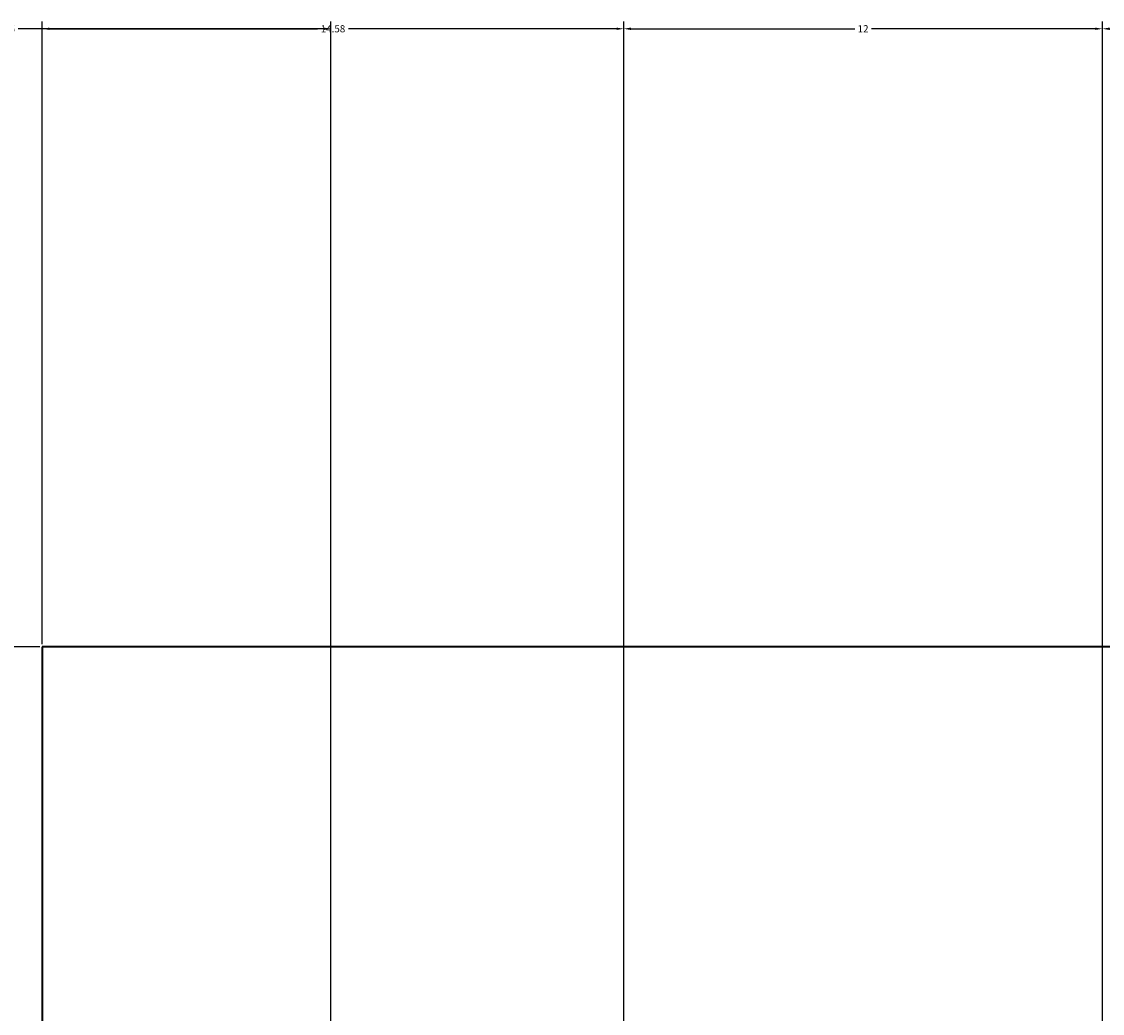
# Model space of a CAD drawing. Units: inches. Extents: x -6 to 289, y -8 to 323.
# Tile 46 of 107: x 19 to 46, y 298 to 323. Entities that reach past the tile are written whole.
import ezdxf

# ---------------------------------------------------------------- set-up
doc = ezdxf.new("R2010")
doc.units = ezdxf.units.IN
doc.header["$MEASUREMENT"] = 0
doc.layers.add('A-ANNO-DIMS', color=2, linetype='Continuous', lineweight=18)
doc.layers.add('A-ELEV', color=7, linetype='Continuous', lineweight=35)
doc.styles.get("Standard").update_dxf_attribs({"font": 'arial.ttf'})
doc.dimstyles.get("Standard").update_dxf_attribs({"dimtxt": 0.18, "dimasz": 0.18, "dimexe": 0.18, "dimexo": 0.0625, "dimgap": 0.09, "dimtad": 0, "dimtih": 1, "dimtoh": 1, "dimdec": 4, "dimzin": 0, "dimdsep": 46, "dimtxsty": 'Standard', "dimcen": 0.09, "dimadec": 0, "dimazin": 0, "dimtfac": 1, "dimtdec": 4, "dimtofl": 0, "dimtmove": 0, "dimatfit": 3, "dimfxl": 1, "dimtolj": 1, "dimtzin": 0, "dimarcsym": 0})

# ---------------------------------------------------------------- blocks, each defined once
blk = doc.blocks.new('*D5')
at = {"layer": 'A-ANNO-DIMS', "color": 0, "lineweight": -2, "transparency": 16777216}
for p, q in [((19.164, 307.351), (19.164, 322.969)), ((19.344, 322.789), (26.068, 322.789)), ((33.564, 322.789), (26.839, 322.789)), ((33.744, 289.105), (33.744, 322.969))]:
    blk.add_line(p, q, dxfattribs=at)
at = {"layer": 'A-ANNO-DIMS', "color": 0, "transparency": 16777216}
for points in [[(19.344, 322.819), (19.344, 322.759), (19.164, 322.789)], [(33.564, 322.819), (33.564, 322.759), (33.744, 322.789)]]:
    blk.add_solid(points, dxfattribs=at)
at = {"layer": 'Defpoints', "color": 0, "transparency": 16777216}
for p in [(33.744, 322.789), (19.164, 307.289), (33.744, 289.043)]:
    blk.add_point(p, dxfattribs=at)
at = {"layer": 'A-ANNO-DIMS', "color": 0, "transparency": 16777216, "insert": (26.454, 322.789), "char_height": 0.18, "attachment_point": 5}
blk.add_mtext('\\A1;14.58', dxfattribs=at)
blk = doc.blocks.new('*D6')
at = {"layer": 'A-ANNO-DIMS', "color": 0, "lineweight": -2, "transparency": 16777216}
for p, q in [((33.744, 289.105), (33.744, 322.969)), ((33.924, 322.789), (39.534, 322.789)), ((45.564, 322.789), (39.953, 322.789)), ((45.744, 277.105), (45.744, 322.969))]:
    blk.add_line(p, q, dxfattribs=at)
at = {"layer": 'A-ANNO-DIMS', "color": 0, "transparency": 16777216}
for points in [[(33.924, 322.819), (33.924, 322.759), (33.744, 322.789)], [(45.564, 322.819), (45.564, 322.759), (45.744, 322.789)]]:
    blk.add_solid(points, dxfattribs=at)
at = {"layer": 'Defpoints', "color": 0, "transparency": 16777216}
for p in [(45.744, 322.789), (33.744, 289.043), (45.744, 277.043)]:
    blk.add_point(p, dxfattribs=at)
at = {"layer": 'A-ANNO-DIMS', "color": 0, "transparency": 16777216, "insert": (39.744, 322.789), "char_height": 0.18, "attachment_point": 5}
blk.add_mtext('\\A1;12', dxfattribs=at)
blk = doc.blocks.new('*D7')
at = {"layer": 'A-ANNO-DIMS', "color": 0, "lineweight": -2, "transparency": 16777216}
for p, q in [((45.744, 277.105), (45.744, 322.969)), ((45.924, 322.789), (66.325, 322.789)), ((87.521, 322.789), (67.119, 322.789)), ((87.701, 277.105), (87.701, 322.969))]:
    blk.add_line(p, q, dxfattribs=at)
at = {"layer": 'A-ANNO-DIMS', "color": 0, "transparency": 16777216}
for points in [[(45.924, 322.819), (45.924, 322.759), (45.744, 322.789)], [(87.521, 322.819), (87.521, 322.759), (87.701, 322.789)]]:
    blk.add_solid(points, dxfattribs=at)
at = {"layer": 'Defpoints', "color": 0, "transparency": 16777216}
for p in [(87.701, 322.789), (45.744, 277.043), (87.701, 277.043)]:
    blk.add_point(p, dxfattribs=at)
at = {"layer": 'A-ANNO-DIMS', "color": 0, "transparency": 16777216, "insert": (66.722, 322.789), "char_height": 0.18, "attachment_point": 5}
blk.add_mtext('\\A1;41.96', dxfattribs=at)
blk = doc.blocks.new('*D21')
at = {"layer": 'A-ANNO-DIMS', "color": 0, "lineweight": -2, "transparency": 16777216}
for p, q in [((19.101, 307.289), (-5.737, 307.289)), ((-5.557, 307.109), (-5.557, 298.348)), ((-5.557, 289.223), (-5.557, 297.984)), ((33.681, 289.043), (-5.737, 289.043))]:
    blk.add_line(p, q, dxfattribs=at)
at = {"layer": 'A-ANNO-DIMS', "color": 0, "transparency": 16777216}
for points in [[(-5.587, 307.109), (-5.527, 307.109), (-5.557, 307.289)], [(-5.587, 289.223), (-5.527, 289.223), (-5.557, 289.043)]]:
    blk.add_solid(points, dxfattribs=at)
at = {"layer": 'Defpoints', "color": 0, "transparency": 16777216}
for p in [(-5.557, 307.289), (19.164, 307.289), (33.744, 289.043)]:
    blk.add_point(p, dxfattribs=at)
at = {"layer": 'A-ANNO-DIMS', "color": 0, "transparency": 16777216, "insert": (-5.557, 298.166), "char_height": 0.18, "attachment_point": 5}
blk.add_mtext('\\A1;18.246', dxfattribs=at)
blk = doc.blocks.new('*D22')
at = {"layer": 'A-ANNO-DIMS', "color": 0, "lineweight": -2, "transparency": 16777216}
for p, q in [((19.101, 307.289), (-5.737, 307.289)), ((-5.557, 307.109), (-5.557, 157.471)), ((-5.557, 7.469), (-5.557, 157.107)), ((11.907, 7.289), (-5.737, 7.289))]:
    blk.add_line(p, q, dxfattribs=at)
at = {"layer": 'A-ANNO-DIMS', "color": 0, "transparency": 16777216}
for points in [[(-5.587, 307.109), (-5.527, 307.109), (-5.557, 307.289)], [(-5.587, 7.469), (-5.527, 7.469), (-5.557, 7.289)]]:
    blk.add_solid(points, dxfattribs=at)
at = {"layer": 'Defpoints', "color": 0, "transparency": 16777216}
for p in [(19.164, 307.289), (-5.557, 7.289), (11.969, 7.289)]:
    blk.add_point(p, dxfattribs=at)
at = {"layer": 'A-ANNO-DIMS', "color": 0, "transparency": 16777216, "insert": (-5.557, 157.289), "char_height": 0.18, "attachment_point": 5}
blk.add_mtext('\\A1;300', dxfattribs=at)
blk = doc.blocks.new('*D27')
at = {"layer": 'A-ANNO-DIMS', "color": 0, "lineweight": -2, "transparency": 16777216}
for p, q in [((19.226, 307.289), (288.653, 307.289)), ((288.473, 307.109), (288.473, 277.471)), ((288.473, 247.469), (288.473, 277.107)), ((247.226, 247.289), (288.653, 247.289))]:
    blk.add_line(p, q, dxfattribs=at)
at = {"layer": 'A-ANNO-DIMS', "color": 0, "transparency": 16777216}
for points in [[(288.443, 307.109), (288.503, 307.109), (288.473, 307.289)], [(288.443, 247.469), (288.503, 247.469), (288.473, 247.289)]]:
    blk.add_solid(points, dxfattribs=at)
at = {"layer": 'Defpoints', "color": 0, "transparency": 16777216}
for p in [(19.164, 307.289), (288.473, 307.289), (247.164, 247.289)]:
    blk.add_point(p, dxfattribs=at)
at = {"layer": 'A-ANNO-DIMS', "color": 0, "transparency": 16777216, "insert": (288.473, 277.289), "char_height": 0.18, "attachment_point": 5}
blk.add_mtext('\\A1;60', dxfattribs=at)
blk = doc.blocks.new('*D57')
at = {"layer": 'A-ANNO-DIMS', "color": 0, "lineweight": -2, "transparency": 16777216}
for p, q in [((9.943, 68.495), (9.943, 322.969)), ((10.123, 322.789), (17.788, 322.789)), ((26.223, 322.789), (18.558, 322.789)), ((26.403, 68.495), (26.403, 322.969))]:
    blk.add_line(p, q, dxfattribs=at)
at = {"layer": 'A-ANNO-DIMS', "color": 0, "transparency": 16777216}
for points in [[(10.123, 322.819), (10.123, 322.759), (9.943, 322.789)], [(26.223, 322.819), (26.223, 322.759), (26.403, 322.789)]]:
    blk.add_solid(points, dxfattribs=at)
at = {"layer": 'Defpoints', "color": 0, "transparency": 16777216}
for p in [(26.403, 322.789), (9.943, 68.432), (26.403, 68.432)]:
    blk.add_point(p, dxfattribs=at)
at = {"layer": 'A-ANNO-DIMS', "color": 0, "transparency": 16777216, "insert": (18.173, 322.789), "char_height": 0.18, "attachment_point": 5}
blk.add_mtext('\\A1;16.46', dxfattribs=at)

msp = doc.modelspace()

# ---------------------------------------------------------------- linework, layer by layer
at = {"layer": 'A-ELEV'}
for p, q in [((19.1638, 307.2888), (19.1638, 68.4322)), ((118.1638, 307.2888), (19.1638, 307.2888))]:
    msp.add_line(p, q, dxfattribs=at)

# ---------------------------------------------------------------- dimensions: what is measured, and where the dimension line sits
at = {"layer": 'A-ANNO-DIMS'}
for base, p1, p2, override, picture, middle in [((26.403, 322.7888), (9.943, 68.4322), (26.403, 68.4322), {"dimdec": 2, "dimlfac": 1, "dimrnd": 0, "dimzin": 0, "dimdsep": 46, "dimlunit": 2}, '*D57', (18.173, 322.7888)), ((33.7437, 322.7888), (19.1638, 307.2888), (33.7437, 289.0427), {"dimdec": 2, "dimlfac": 1, "dimrnd": 0, "dimzin": 0, "dimdsep": 46, "dimlunit": 2}, '*D5', (26.4537, 322.7888)), ((45.7437, 322.7888), (33.7437, 289.0427), (45.7437, 277.0427), {"dimdec": 0, "dimlfac": 1, "dimrnd": 0, "dimzin": 0, "dimdsep": 46, "dimlunit": 2}, '*D6', (39.7437, 322.7888)), ((87.7007, 322.7888), (45.7437, 277.0427), (87.7007, 277.0427), {"dimdec": 2, "dimlfac": 1, "dimrnd": 0, "dimzin": 0, "dimdsep": 46, "dimlunit": 2}, '*D7', (66.7222, 322.7888))]:
    dim = msp.add_linear_dim(base=base, p1=p1, p2=p2, dimstyle='Standard', override=override, dxfattribs=at)
    dim.commit()
    dim.dimension.update_dxf_attribs({"geometry": picture, "text_midpoint": middle})
for base, p1, p2, override, picture, middle in [((-5.557, 307.2888), (33.7437, 289.0427), (19.1638, 307.2888), {"dimdec": 3, "dimlfac": 1, "dimrnd": 0, "dimzin": 0, "dimdsep": 46, "dimlunit": 2}, '*D21', (-5.557, 298.1657)), ((-5.557, 7.2888), (19.1638, 307.2888), (11.9692, 7.2888), {"dimdec": 0, "dimlfac": 1, "dimrnd": 0, "dimzin": 0, "dimdsep": 46, "dimlunit": 2}, '*D22', (-5.557, 157.2888)), ((288.4733, 307.2888), (247.1638, 247.2888), (19.1638, 307.2888), {"dimdec": 0, "dimlfac": 1, "dimrnd": 0, "dimzin": 0, "dimdsep": 46, "dimlunit": 2}, '*D27', (288.4733, 277.2888))]:
    dim = msp.add_linear_dim(base=base, p1=p1, p2=p2, angle=90, dimstyle='Standard', override=override, dxfattribs=at)
    dim.commit()
    dim.dimension.update_dxf_attribs({"geometry": picture, "text_midpoint": middle})

doc.saveas('drawing.dxf')
